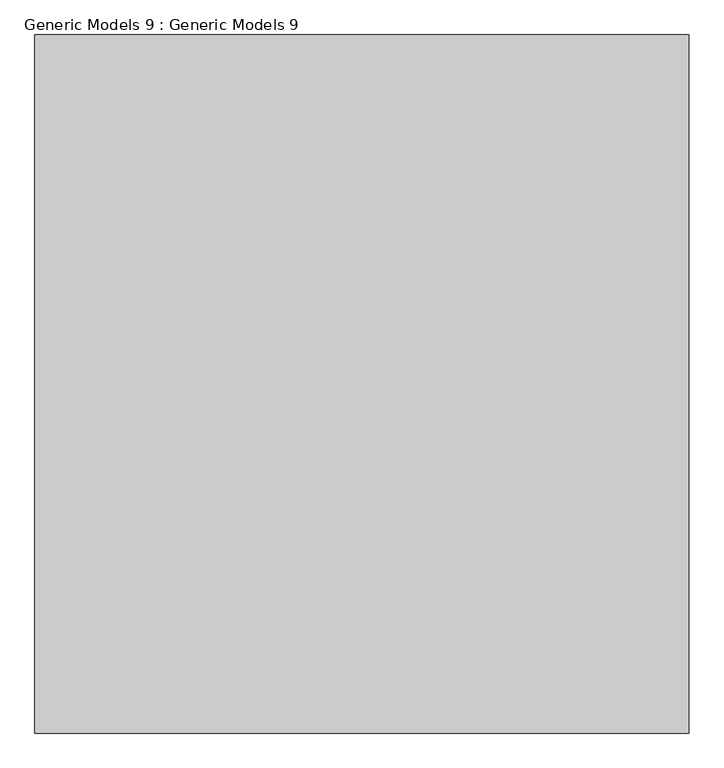
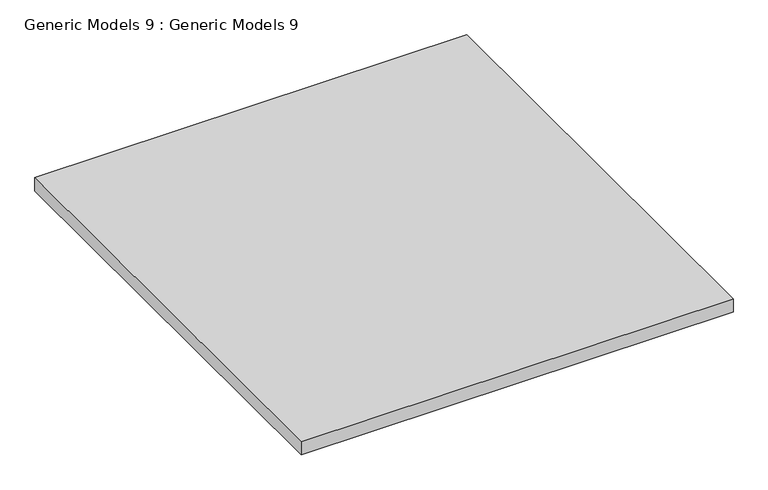
"""IFC4 building model written with IfcOpenShell, lengths in millimetres: proxy geometry, Generic Models 9 : Generic Models 9."""

from ifc_helpers import new_model, si_unit, frame, origin, place, context, project, spatial, polyline, outline, extrude, source, transform, mapped, element, save


def generic_models_9_generic_models_9_3f232281(model_context):
    return source(origin(), model_context, "Body", "SweptSolid", [
        extrude(outline(polyline([(-162.4586008, -7335.6844117), (-4912.2586008, -7335.6844117), (-4912.2586008, -2268.3844117), (-162.4586008, -2268.3844117), (-162.4586008, -7335.6844117)])), frame((0.0, 0.0, 2895.6), z_axis=(0.0, 0.0, 1.0), x_axis=(1.0, 0.0, 0.0)), (0.0, 0.0, 1.0), 152.4),
    ])


if __name__ == "__main__":
    model = new_model("IFC4")
    model_context = context("Model", 3, world=origin())
    ifc_project = project(units=[si_unit("LENGTHUNIT", "METRE", prefix="MILLI")], contexts=[model_context])
    site = spatial("IfcSite", under=ifc_project)
    building = spatial("IfcBuilding", under=site)
    placement = place(None, origin())
    generic_models_9_generic_models_9_shape = generic_models_9_generic_models_9_3f232281(model_context)
    element("IfcBuildingElementProxy", 1, Name="Generic Models 9 : Generic Models 9", ObjectType="Generic Models 9 : Generic Models 9", at=placement, inside=building, context=model_context, shape_type="MappedRepresentation", body=[
        mapped(generic_models_9_generic_models_9_shape, transform((0.0, 0.0, 0.0), x_axis=(1.0, 0.0, 0.0), y_axis=(0.0, 1.0, 0.0), z_axis=(0.0, 0.0, 1.0))),
    ])
    save(model, "model.ifc")

# Revit data of these elements
# Element 1 (IfcBuildingElementProxy, "Generic Models 9 : Generic Models 9")
#   Materials on its faces: "wood ceiling"
# Materials
#   "wood ceiling": class "Generic", colour RGB 120 120 120, transparency 0, Cost = 0
